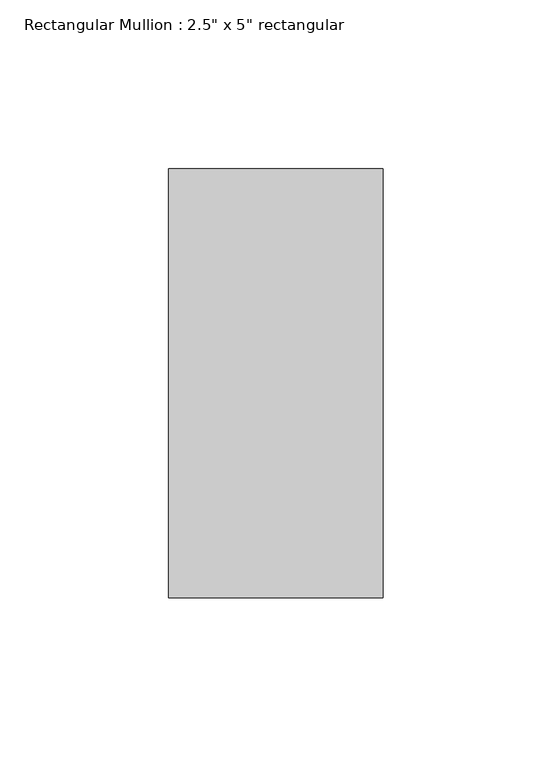
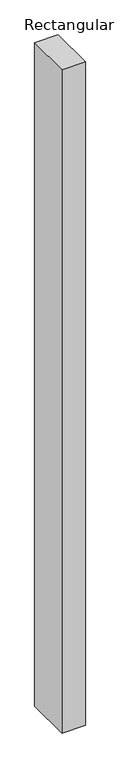
"""IFC4 building model written with IfcOpenShell, lengths in millimetres: member geometry."""

from ifc_helpers import new_model, si_unit, frame, origin, place, context, project, spatial, polyline, outline, extrude, source, transform, mapped, element, save


def member_c78e4eb6(model_context):
    return source(origin(), model_context, "Body", "SweptSolid", [
        extrude(outline(polyline([(0.0, 63.5), (0.0, -63.5), (-63.5, -63.5), (-63.5, 63.5), (0.0, 63.5)])), frame((0.0, 0.0, -1896.5759417), z_axis=(0.0, 0.0, 1.0), x_axis=(1.0, 0.0, 0.0)), (0.0, 0.0, 1.0), 1896.5759417),
    ])


if __name__ == "__main__":
    model = new_model("IFC4")
    model_context = context("Model", 3, world=origin())
    ifc_project = project(units=[si_unit("LENGTHUNIT", "METRE", prefix="MILLI")], contexts=[model_context])
    site = spatial("IfcSite", under=ifc_project)
    building = spatial("IfcBuilding", under=site)
    placement = place(None, origin())
    member_shape = member_c78e4eb6(model_context)
    element("IfcMember", 1, ObjectType="Rectangular Mullion : 2.5\" x 5\" rectangular", at=placement, inside=building, context=model_context, shape_type="MappedRepresentation", body=[
        mapped(member_shape, transform((0.0, 0.0, 0.0), x_axis=(1.0, 0.0, 0.0), y_axis=(0.0, 1.0, 0.0), z_axis=(0.0, 0.0, 1.0))),
    ])
    save(model, "model.ifc")

# Revit data of these elements
# Type "Rectangular Mullion : 2.5\" x 5\" rectangular"
#   built-in parameter 1007304 = 0.416667 (stored number, unit not read)
#   built-in parameter 1007301 = 0.104167 (stored number, unit not read)
#   built-in parameter 1007300 = 0.104167 (stored number, unit not read)
# Element 1 (IfcMember, "Rectangular Mullion : 2.5\" x 5\" rectangular")
#   Materials on its faces: "Iron, Ductile"
# Materials
#   "Iron, Ductile": class "Metal", colour RGB 0 0 0, transparency 0, Description = "Ductile cast iron", Cost = 0
